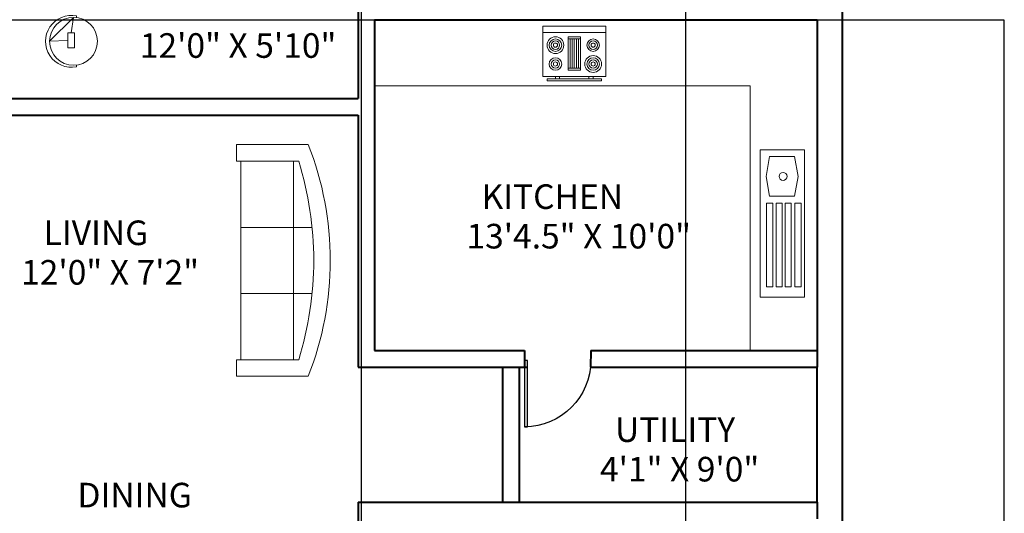
# Model space of a CAD drawing. Units: inches. Extents: x -46 to 1145, y -527 to 760.
# Tile 20 of 57: x 788 to 1145, y -218 to -39. Entities that reach past the tile are written whole.
import ezdxf

# ---------------------------------------------------------------- set-up
doc = ezdxf.new("R2010")
doc.units = ezdxf.units.IN
doc.header["$MEASUREMENT"] = 0
for name, color, linetype, lineweight in [('A-ANNO-DIMS', 2, 'Continuous', 18), ('A-AREA-IDEN', 1, 'Continuous', 18), ('A-EQPM', 2, 'Continuous', 18), ('A-FLOR-CASE', 32, 'Continuous', 18), ('A-FLOR-FIXT', 9, 'Continuous', 18), ('A-FURN', 2, 'Continuous', 13), ('DOORS', 3, 'Continuous', 25), ('WALLS', 4, 'Continuous', 40)]:
    doc.layers.add(name, color=color, linetype=linetype, lineweight=lineweight)
doc.styles.get("Standard").update_dxf_attribs({"font": 'arial.ttf'})
doc.dimstyles.get("Standard").update_dxf_attribs({"dimtxt": 0.18, "dimasz": 0.18, "dimexe": 0.18, "dimexo": 0.0625, "dimgap": 0.09, "dimtad": 0, "dimtih": 1, "dimtoh": 1, "dimdec": 0, "dimzin": 0, "dimdsep": 46, "dimlunit": 3, "dimtxsty": 'Standard', "dimcen": 0.09, "dimadec": 0, "dimazin": 0, "dimtfac": 1, "dimtdec": 0, "dimtofl": 0, "dimtmove": 0, "dimatfit": 3, "dimfxl": 1, "dimtolj": 1, "dimtzin": 0, "dimarcsym": 0})

# ---------------------------------------------------------------- blocks, each defined once
blk = doc.blocks.new('*U2')
for p, q in [((0, 0), (0, -6)), ((40, 0), (40, -6))]:
    blk.add_line(p, q)
blk.add_lwpolyline([(0, 0), (0, 40), (1.75, 40), (1.75, 0)], close=True)
blk.add_arc((0, 0), 40, 0, 90)
blk = doc.blocks.new('Range-Oven - 30 in top')
for p, q in [((0, -3), (30, -3)), ((12, -6), (18, -6)), ((13, -20), (13, -6)), ((14, -6), (14, -20)), ((15, -20), (15, -6)), ((16, -6), (16, -20)), ((17, -20), (17, -6)), ((18, -20), (12, -20)), ((6, -24), (6, -25)), ((8, -25), (8, -24)), ((22, -25), (22, -24)), ((24, -24), (24, -25))]:
    blk.add_line(p, q)
for points in [[(0, -24), (0, 0), (30, 0), (30, -24)], [(12, -21), (12, -5), (18, -5), (18, -21)], [(2, -26), (2, -25), (28, -25), (28, -26)]]:
    blk.add_lwpolyline(points, close=True)
for centre, radius in [((6, -9), 4), ((6, -9), 3), ((6, -9), 2), ((6, -9), 1), ((24, -9), 3), ((24, -9), 2), ((24, -9), 1), ((24, -18), 4), ((6, -18), 3), ((6, -18), 2), ((6, -18), 1), ((24, -18), 3), ((24, -18), 2), ((24, -18), 1)]:
    blk.add_circle(centre, radius)
blk = doc.blocks.new('Sofa - Roundback 7 ft.')
for p, q in [((-12.00002, -32.4421), (-12.00003, -6.5971)), ((11.99997, -32.4421), (11.99998, -6.5971)), ((-36.000027, -34), (-36.000027, -11.4696)), ((-35.999844, -13.3819), (35.9998, -13.3819)), ((35.99998, -34), (35.99998, -11.4696)), ((-36.000027, -32.4421), (35.99998, -32.4421))]:
    blk.add_line(p, q)
for points in [[(-36.000027, -34), (-42.000027, -34), (-42.000027, -8)], [(41.99998, -8), (41.99998, -34), (35.99998, -34)]]:
    blk.add_lwpolyline(points)
for centre, radius, start, end in [((0, -114.25), 114.25, 68.43141, 111.5686), ((-0.00001, -127.1968), 121.1968, 72.72033, 107.2797)]:
    blk.add_arc(centre, radius, start, end)
blk = doc.blocks.new('SINK-DRAINBOARD')
for p, q in [((3.38, 50.9), (2.09, 43.74)), ((12.47, 50.9), (13.77, 43.74)), ((3.38, 36.58), (2.09, 43.74)), ((12.47, 36.58), (13.77, 43.74))]:
    blk.add_line(p, q)
for points in [[(16.07, 0), (0, 0), (0, 53.35), (16.07, 53.35)], [(4.51, 3.73), (2.3, 3.73), (2.3, 34.08), (4.51, 34.08)], [(7.92, 3.73), (5.72, 3.73), (5.72, 34.08), (7.92, 34.08)], [(11.26, 3.73), (9.05, 3.73), (9.05, 34.08), (11.26, 34.08)], [(14.8, 3.73), (12.59, 3.73), (12.59, 34.08), (14.8, 34.08)]]:
    blk.add_lwpolyline(points, close=True)
for points in [[(3.38, 50.9), (12.47, 50.9)], [(12.47, 36.58), (3.38, 36.58)]]:
    blk.add_lwpolyline(points)
blk.add_circle((8.28, 43.74), 1.44)
blk = doc.blocks.new('BALCONY-CHAIR')
for p, q in [((1.49, 9.38), (10.16, 18.05)), ((9.33, 12.41), (10.16, 18.05)), ((11.28, 17.97), (11.28, 18.57)), ((8.08, 9.69), (1.49, 9.38)), ((11.2, 0.17), (11.2, 0.77))]:
    blk.add_line(p, q)
blk.add_lwpolyline([(10.57, 6.97), (8.08, 6.97), (8.08, 12.41), (10.57, 12.41)], close=True)
blk.add_circle((10.16, 9.38), 8.67)
blk.add_arc((9.38, 9.38), 9.38, 78.3491, 281.1485)
blk = doc.blocks.new('KITCHEN-COUNTER-L')
for p, q in [((136.17, 96), (0, 96)), ((136.17, 24), (136.17, 96)), ((136.17, 0), (136.17, 24))]:
    blk.add_line(p, q)
blk = doc.blocks.new('*D694')
at = {"layer": 'A-ANNO-DIMS', "color": 0, "lineweight": -2, "transparency": 16777216}
for p, q in [((912.18, 101.46), (912.18, -527.26)), ((1029.77, 101.46), (1029.77, -527.26)), ((912.36, -527.08), (970.59, -527.08)), ((1029.59, -527.08), (971.36, -527.08))]:
    blk.add_line(p, q, dxfattribs=at)
at = {"layer": 'A-ANNO-DIMS', "color": 0, "transparency": 16777216}
for points in [[(912.36, -527.05), (912.36, -527.11), (912.18, -527.08)], [(1029.59, -527.05), (1029.59, -527.11), (1029.77, -527.08)]]:
    blk.add_solid(points, dxfattribs=at)
at = {"layer": 'Defpoints', "color": 0, "transparency": 16777216}
for p in [(912.18, 101.52), (1029.77, 101.52), (1029.77, -527.08)]:
    blk.add_point(p, dxfattribs=at)
at = {"layer": 'A-ANNO-DIMS', "color": 0, "transparency": 16777216, "insert": (970.97, -527.08), "char_height": 0.18, "attachment_point": 5}
blk.add_mtext('\\A1;117.6', dxfattribs=at)
blk = doc.blocks.new('*D702')
at = {"layer": 'A-ANNO-DIMS', "color": 0, "lineweight": -2, "transparency": 16777216}
for p, q in [((189.63, -39.48), (1145.34, -39.48)), ((1145.16, -39.66), (1145.16, -249.3)), ((1145.16, -459.3), (1145.16, -249.66)), ((183.63, -459.48), (1145.34, -459.48))]:
    blk.add_line(p, q, dxfattribs=at)
at = {"layer": 'A-ANNO-DIMS', "color": 0, "transparency": 16777216}
for points in [[(1145.13, -39.66), (1145.19, -39.66), (1145.16, -39.48)], [(1145.13, -459.3), (1145.19, -459.3), (1145.16, -459.48)]]:
    blk.add_solid(points, dxfattribs=at)
at = {"layer": 'Defpoints', "color": 0, "transparency": 16777216}
for p in [(189.56, -39.48), (1145.16, -39.48), (183.56, -459.48)]:
    blk.add_point(p, dxfattribs=at)
at = {"layer": 'A-ANNO-DIMS', "color": 0, "transparency": 16777216, "insert": (1145.16, -249.48), "char_height": 0.18, "attachment_point": 5}
blk.add_mtext('\\A1;420', dxfattribs=at)

msp = doc.modelspace()

# ---------------------------------------------------------------- linework, layer by layer
at = {"layer": 'WALLS'}
for p, q in [((911.0637, -30.4824), (911.0637, -68.1114)), ((1086.5637, -30.4824), (1086.5637, -468.4824)), ((917.0637, -39.4824), (917.0637, -159.4824)), ((917.0637, -39.4824), (1077.5637, -39.4824)), ((1077.5637, -39.4824), (1077.5637, -165.4824)), ((761.0637, -68.1114), (911.0637, -68.1114)), ((761.0637, -74.1114), (911.0637, -74.1114)), ((911.0637, -74.1114), (911.0637, -165.4824)), ((917.0637, -159.4824), (971.4282, -159.4824)), ((971.4282, -159.4824), (971.4282, -165.4824)), ((995.4282, -159.4824), (995.3079, -165.4824)), ((995.4282, -159.4824), (1077.5637, -159.4824)), ((911.0637, -165.4824), (972.4782, -165.4824)), ((963.5637, -214.4824), (963.5637, -165.4824)), ((969.5637, -214.4824), (969.5637, -165.4824)), ((995.3079, -165.4824), (1077.5637, -165.4824)), ((1077.5637, -214.4824), (1077.5637, -165.4824)), ((911.0637, -214.4824), (911.0637, -322.768)), ((911.0637, -214.4824), (1077.5637, -214.4824)), ((1077.5637, -214.4824), (1077.5637, -220.4824))]:
    msp.add_line(p, q, dxfattribs=at)

# ---------------------------------------------------------------- block references
at = {"layer": 'A-EQPM', "xscale": 0.7600381531222953, "yscale": 0.7600381531222953, "zscale": 0.7600381531222953}
msp.add_blockref('Range-Oven - 30 in top', (978.0568, -41.8749), dxfattribs=at)
at = {"layer": 'A-FLOR-CASE'}
msp.add_blockref('KITCHEN-COUNTER-L', (917.064, -159.482), dxfattribs=at)
at = {"layer": 'A-FLOR-FIXT'}
msp.add_blockref('SINK-DRAINBOARD', (1056.873, -140.056), dxfattribs=at)
at = {"layer": 'A-FURN'}
msp.add_blockref('BALCONY-CHAIR', (797.7165, -56.7085), dxfattribs=at)
at = {"layer": 'A-FURN', "rotation": 270}
msp.add_blockref('Sofa - Roundback 7 ft.', (900.983, -126.7903), dxfattribs=at)
at = {"layer": 'DOORS', "xscale": -0.6, "yscale": 0.6, "zscale": 0.6, "rotation": 180}
msp.add_blockref('*U2', (971.4282, -163.0824), dxfattribs=at)

# ---------------------------------------------------------------- texts
at = {"layer": 'A-AREA-IDEN'}
for s, height, p in [('12\'0" X 5\'10"', 8.923264, (831.917, -53.3134)), ('  KITCHEN', 8.92326, (950.3531, -108.1155)), ('   LIVING', 8.92326, (788.8696, -121.2284)), ('13\'4.5" X 10\'0"', 8.923264, (950.3531, -122.4499)), ('12\'0" X 7\'2"', 8.923264, (788.8696, -135.5628)), ('   UTILITY', 8.92326, (996.0384, -192.6176)), (' 4\'1" X 9\'0"', 8.923264, (996.0384, -206.9521)), ('   DINING', 8.92326, (801.1059, -216.3591))]:
    msp.add_text(s, height=height, dxfattribs=at).set_placement(p)

# ---------------------------------------------------------------- dimensions: what is measured, and where the dimension line sits
at = {"layer": 'A-ANNO-DIMS'}
dim = msp.add_linear_dim(base=(1029.7714, -527.0824), p1=(912.1762, 101.5176), p2=(1029.7714, 101.5176), dimstyle='Standard', override={"dimdec": 1, "dimlfac": 1, "dimrnd": 0, "dimzin": 0, "dimdsep": 46, "dimlunit": 2}, dxfattribs=at)
dim.commit()
dim.dimension.update_dxf_attribs({"geometry": '*D694', "text_midpoint": (970.9738, -527.0824)})
dim = msp.add_linear_dim(base=(1145.1637, -39.4824), p1=(183.5637, -459.4824), p2=(189.5637, -39.4824), angle=90, dimstyle='Standard', override={"dimdec": 0, "dimlfac": 1, "dimrnd": 0, "dimzin": 0, "dimdsep": 46, "dimlunit": 2}, dxfattribs=at)
dim.commit()
dim.dimension.update_dxf_attribs({"geometry": '*D702', "text_midpoint": (1145.1637, -249.4824)})

doc.saveas('drawing.dxf')
